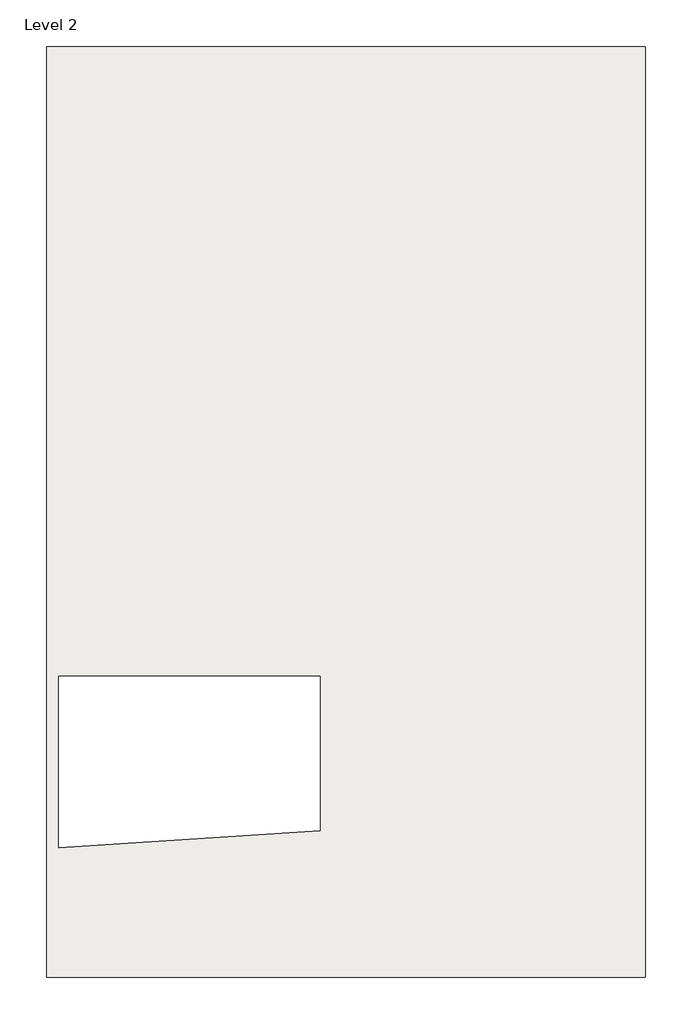
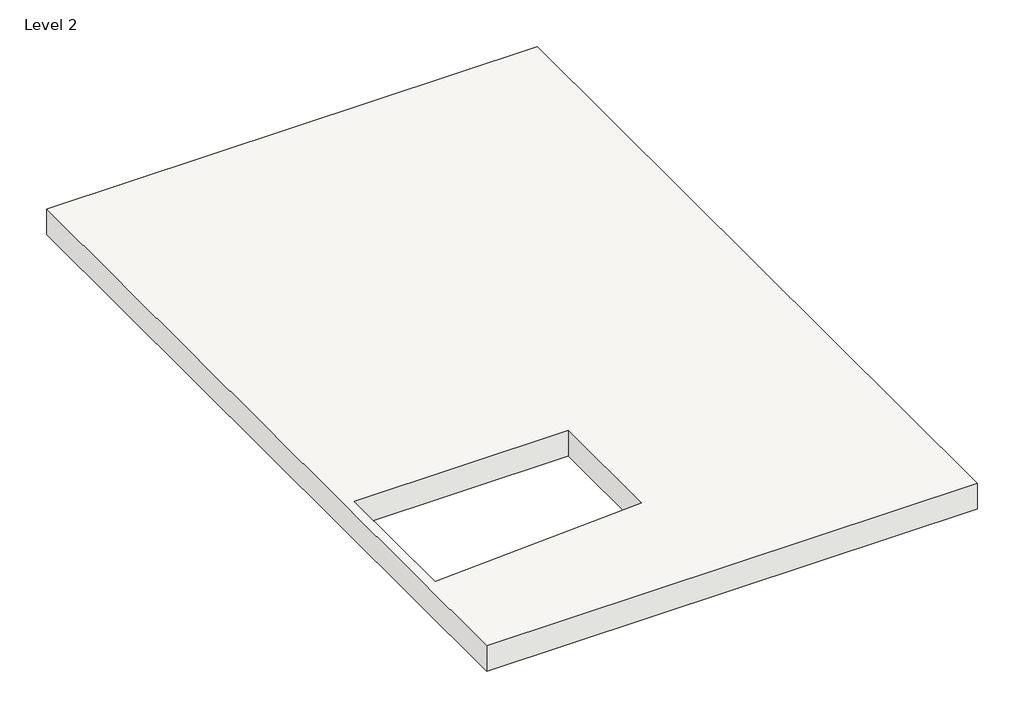
# One storey: 1 roof.
"""IFC4 building model written with IfcOpenShell, lengths in millimetres."""

from ifc_helpers import new_model, si_unit, frame, origin, place, context, project, spatial, polyline, outline, extrude, element, save

model = new_model("IFC4")

# Units and contexts
model_context = context("Model", 3, world=origin())
ifc_project = project(units=[si_unit("LENGTHUNIT", "METRE", prefix="MILLI")], contexts=[model_context])

# Site, building, storey
site = spatial("IfcSite", under=ifc_project)
building = spatial("IfcBuilding", under=site)
storey = spatial("IfcBuildingStorey", under=building, Name="Level 2", Elevation=3048.0)

# Roof
placement = place(None, origin())
element("IfcRoof", 1, ObjectType="Steel Truss - Insulation on Metal Deck - EPDM", at=placement, inside=storey, context=model_context, shape_type="SweptSolid", body=[
    extrude(outline(polyline([(-7299.1957152, 16067.7691167), (2657.6042848, 16067.7691167), (2657.6042848, 599.1691167), (-7299.1957152, 599.1691167), (-7299.1957152, 16067.7691167)]), holes=[polyline([(-7095.9957152, 2758.1691167), (-2752.5957152, 3036.4892317), (-2752.5957152, 5602.9691167), (-7095.9957152, 5602.9691167), (-7095.9957152, 2758.1691167)])]), frame((0.0, 0.0, 3048.0), z_axis=(0.0, 0.0, 1.0), x_axis=(1.0, 0.0, 0.0)), (0.0, 0.0, 1.0), 546.1),
])

save(model, "model.ifc")

# Revit data of these elements
# Type "Steel Truss - Insulation on Metal Deck - EPDM"
#   Assembly Code = "B1020"
#   Layers, outside or top first: 0' - 0 1/4" "Roofing, EPDM Membrane" (function 4); 0' - 5" "Rigid insulation" (function 3); 0' - 0 1/4" "Metal Deck" (function 1); 1' - 4" "Structure, Steel Bar Joist Layer" (function 1)
# Element 1 (IfcRoof, "Steel Truss - Insulation on Metal Deck - EPDM")
#   built-in parameter 1001705 = 11.7917 (stored number, unit not read)
#   built-in parameter 1001710 = 33615
#   Phase Created = New Construction
#   Materials on its faces: "Structure, Steel Bar Joist Layer", "Roofing, EPDM Membrane"
# Materials
#   "Roofing, EPDM Membrane": class "Generic", colour RGB 127 127 127, transparency 0, Description = "EPDM roof membrane", Cost = 0
#   "Rigid insulation": class "Generic", colour RGB 127 127 127, transparency 0, Description = "Rigid foam insulation board", Cost = 0
#   "Metal Deck": class "Metal", colour RGB 199 199 199, transparency 0, Description = "Steel, mill finish", Cost = 0
#   "Structure, Steel Bar Joist Layer": class "Metal", colour RGB 127 127 127, transparency 0, Description = "Bar joists, thermal airspace", Cost = 0
